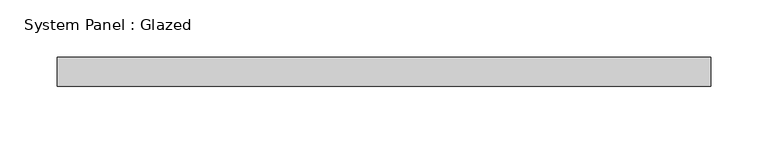
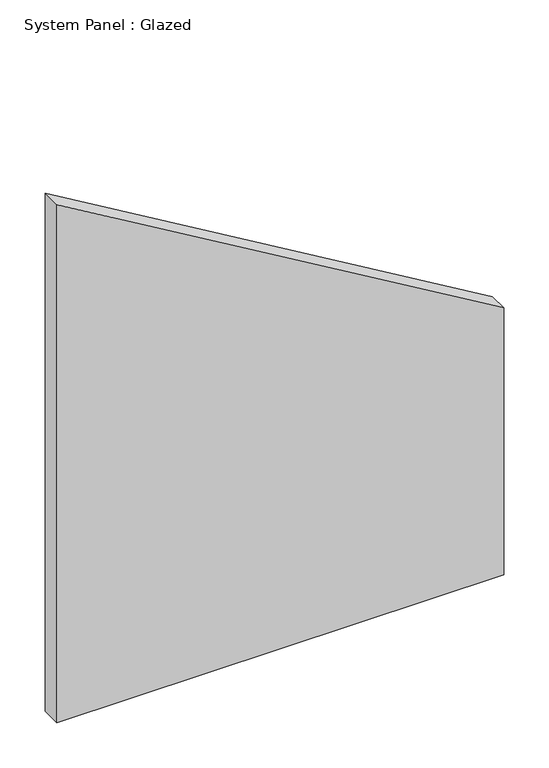
"""IFC4 building model written with IfcOpenShell, lengths in millimetres: plate geometry, System Panel : Glazed."""

from ifc_helpers import new_model, si_unit, frame, origin, place, context, project, spatial, polyline, outline, extrude, source, transform, mapped, element, save


def system_panel_glazed_9c640d8a(model_context):
    return source(origin(), model_context, "Body", "SweptSolid", [
        extrude(outline(polyline([(0.0, -285.75), (0.0, 285.75), (360.6432431, 285.75), (700.3109514, -285.75), (0.0, -285.75)])), frame((0.0, 19.05, 0.0), z_axis=(0.0, 1.0, 0.0), x_axis=(0.0, 0.0, 1.0)), (0.0, 0.0, 1.0), 25.4),
    ])


if __name__ == "__main__":
    model = new_model("IFC4")
    model_context = context("Model", 3, world=origin())
    ifc_project = project(units=[si_unit("LENGTHUNIT", "METRE", prefix="MILLI")], contexts=[model_context])
    site = spatial("IfcSite", under=ifc_project)
    building = spatial("IfcBuilding", under=site)
    placement = place(None, origin())
    system_panel_glazed_shape = system_panel_glazed_9c640d8a(model_context)
    element("IfcPlate", 1, ObjectType="System Panel : Glazed", at=placement, inside=building, context=model_context, shape_type="MappedRepresentation", body=[
        mapped(system_panel_glazed_shape, transform((0.0, 0.0, 0.0), x_axis=(1.0, 0.0, 0.0), y_axis=(0.0, 1.0, 0.0), z_axis=(0.0, 0.0, 1.0))),
    ])
    save(model, "model.ifc")

# Revit data of these elements
# Type "System Panel : Glazed"
#   Construction Type Id = "GSP4R"
#   Analytic Construction = "1/8 in Pilkington single glazing"
#   Visual Light Transmittance = 0.9
#   Solar Heat Gain Coefficient = 0.86
#   Heat Transfer Coefficient (U) = 1.18115 BTU/(h·ft²·°F)
#   Define Thermal Properties by = 1
# Element 1 (IfcPlate, "System Panel : Glazed")
#   Materials on its faces: "Glass"
# Materials
#   "Glass": class "Glass", colour RGB 0 128 192, transparency 0.75, Description = "Soda Lime Glass", Cost = 0
